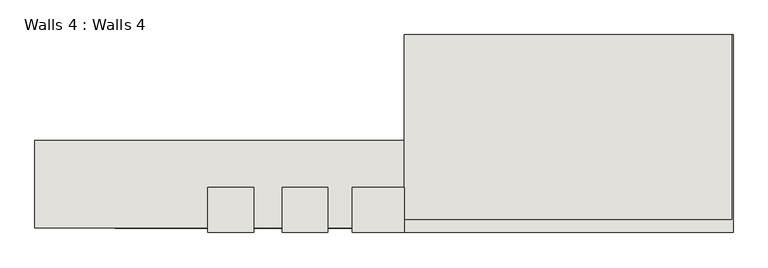
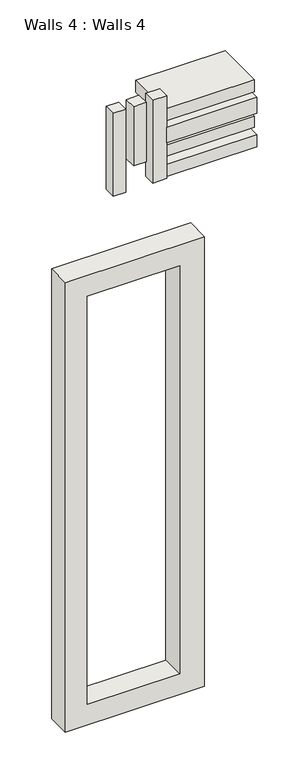
"""IFC4 building model written with IfcOpenShell, lengths in millimetres: wall geometry, Walls 4 : Walls 4."""

from ifc_helpers import new_model, si_unit, frame, origin, place, context, project, spatial, polyline, outline, extrude, source, transform, mapped, element, save


def walls_4_walls_4_15621a10(model_context):
    return source(origin(), model_context, "Body", "SweptSolid", [
        extrude(outline(polyline([(-10973.3513569, 891.6548743), (-9886.3455363, 891.6548743), (-9886.3455363, 233.8331416), (-10973.3513569, 233.8331416), (-10973.3513569, 891.6548743)])), frame((0.0, 0.0, 11455.4), z_axis=(0.0, 0.0, 1.0), x_axis=(1.0, 0.0, 0.0)), (0.0, 0.0, 1.0), 152.4),
        extrude(outline(polyline([(-10979.7013569, 891.6548743), (-9885.6159901, 891.6548743), (-9885.6159901, 234.1737812), (-10979.7013569, 234.1737812), (-10979.7013569, 891.6548743)])), frame((0.0, 0.0, 11887.5408216), z_axis=(0.0, 0.0, 1.0), x_axis=(1.0, 0.0, 0.0)), (0.0, 0.0, 1.0), 203.0271636),
        extrude(outline(polyline([(-10979.7013569, 891.6548743), (-9889.4803394, 891.6548743), (-9889.4803394, 277.4383022), (-10979.7013569, 277.4383022), (-10979.7013569, 891.6548743)])), frame((0.0, 0.0, 12141.2), z_axis=(0.0, 0.0, 1.0), x_axis=(1.0, 0.0, 0.0)), (0.0, 0.0, 1.0), 152.4),
        extrude(outline(polyline([(-10979.7013569, 891.6548743), (-9888.4651845, 891.6548743), (-9888.4651845, 277.4383022), (-10979.7013569, 277.4383022), (-10979.7013569, 891.6548743)])), frame((0.0, 0.0, 11683.2026091), z_axis=(0.0, 0.0, 1.0), x_axis=(1.0, 0.0, 0.0)), (0.0, 0.0, 1.0), 138.5452884),
        extrude(outline(polyline([(10508.7650496, -10513.5899541), (10508.7650496, -12207.3340235), (4717.5650496, -12207.3340235), (4717.5650496, -10513.5899541), (10508.7650496, -10513.5899541)]), holes=[polyline([(10242.8350501, -10815.9776586), (4985.0350501, -10815.9776586), (4985.0350501, -11940.8518902), (10242.8350501, -11940.8518902), (10242.8350501, -10815.9776586)])]), frame((0.0, 248.8111976, 0.0), z_axis=(0.0, 1.0, 0.0), x_axis=(0.0, 0.0, 1.0)), (0.0, 0.0, 1.0), 291.5977638),
        extrude(outline(polyline([(-11632.1844908, 383.6548743), (-11479.7844908, 383.6548743), (-11479.7844908, 234.1737812), (-11632.1844908, 234.1737812), (-11632.1844908, 383.6548743)])), frame((0.0, 0.0, 11430.0), z_axis=(0.0, 0.0, 1.0), x_axis=(1.0, 0.0, 0.0)), (0.0, 0.0, 1.0), 1066.8),
        extrude(outline(polyline([(-11385.3171605, 383.6548743), (-11232.9171605, 383.6548743), (-11232.9171605, 234.1737812), (-11385.3171605, 234.1737812), (-11385.3171605, 383.6548743)])), frame((0.0, 0.0, 11734.8), z_axis=(0.0, 0.0, 1.0), x_axis=(1.0, 0.0, 0.0)), (0.0, 0.0, 1.0), 762.0),
        extrude(outline(polyline([(-11152.2129499, 383.6548743), (-10979.7013569, 383.6548743), (-10979.7013569, 234.1737812), (-11152.2129499, 234.1737812), (-11152.2129499, 383.6548743)])), frame((0.0, 0.0, 11430.0), z_axis=(0.0, 0.0, 1.0), x_axis=(1.0, 0.0, 0.0)), (0.0, 0.0, 1.0), 1066.8),
    ])


if __name__ == "__main__":
    model = new_model("IFC4")
    model_context = context("Model", 3, world=origin())
    ifc_project = project(units=[si_unit("LENGTHUNIT", "METRE", prefix="MILLI")], contexts=[model_context])
    site = spatial("IfcSite", under=ifc_project)
    building = spatial("IfcBuilding", under=site)
    placement = place(None, origin())
    walls_4_walls_4_shape = walls_4_walls_4_15621a10(model_context)
    element("IfcWall", 1, ObjectType="Walls 4 : Walls 4", at=placement, inside=building, context=model_context, shape_type="MappedRepresentation", body=[
        mapped(walls_4_walls_4_shape, transform((0.0, 0.0, 0.0), x_axis=(1.0, 0.0, 0.0), y_axis=(0.0, 1.0, 0.0), z_axis=(0.0, 0.0, 1.0))),
    ])
    save(model, "model.ifc")

# Revit data of these elements
# Element 1 (IfcWall, "Walls 4 : Walls 4")
#   Materials on its faces: "Default Wall"
# Materials
#   "Default Wall": colour RGB 128 128 128, transparency 0
